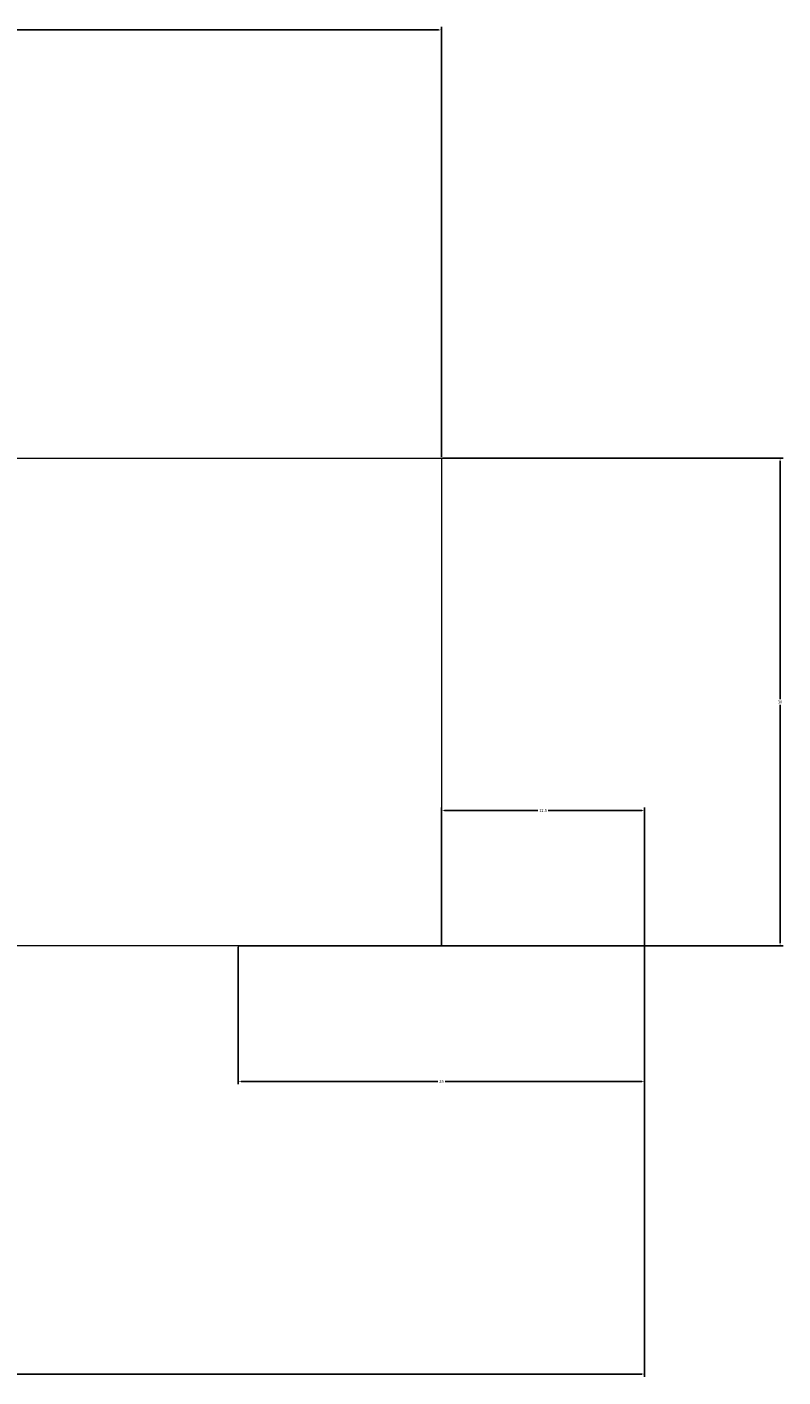
# Model space of a CAD drawing. Units: millimetres. Extents: x 2117 to 2298, y 1328 to 1411.
# Tile 3 of 3: x 2252 to 2298, y 1328 to 1411. Entities that reach past the tile are written whole.
import ezdxf

# ---------------------------------------------------------------- set-up
doc = ezdxf.new("R2010")
doc.units = ezdxf.units.MM
doc.layers.add('M-CONS', color=8, linetype='Continuous', lineweight=18)
doc.layers.add('M-DIMS', color=2, linetype='Continuous', lineweight=18)
doc.styles.get("Standard").update_dxf_attribs({"font": 'arial.ttf'})
doc.dimstyles.get("Standard").update_dxf_attribs({"dimtxt": 0.18, "dimasz": 0.18, "dimexe": 0.18, "dimexo": 0.0625, "dimgap": 0.09, "dimtad": 0, "dimtih": 1, "dimtoh": 1, "dimdec": 4, "dimzin": 0, "dimdsep": 46, "dimtxsty": 'Standard', "dimcen": 0.09, "dimadec": 0, "dimazin": 0, "dimtfac": 1, "dimtdec": 4, "dimtofl": 0, "dimtmove": 0, "dimatfit": 3, "dimfxl": 1, "dimtolj": 1, "dimtzin": 0, "dimarcsym": 0})

# ---------------------------------------------------------------- blocks, each defined once
blk = doc.blocks.new('*D7')
at = {"layer": 'Defpoints', "color": 0, "transparency": 16777216}
for p in [(2277.416, 1411.113), (2205.416, 1384.783), (2277.416, 1384.783)]:
    blk.add_point(p, dxfattribs=at)
at = {"layer": 'M-DIMS', "color": 0, "lineweight": -2, "transparency": 16777216}
for p, q in [((2205.416, 1384.845), (2205.416, 1411.293)), ((2205.596, 1411.113), (2241.199, 1411.113)), ((2277.236, 1411.113), (2241.633, 1411.113)), ((2277.416, 1384.845), (2277.416, 1411.293))]:
    blk.add_line(p, q, dxfattribs=at)
at = {"layer": 'M-DIMS', "color": 0, "transparency": 16777216}
for points in [[(2205.596, 1411.143), (2205.596, 1411.083), (2205.416, 1411.113)], [(2277.236, 1411.143), (2277.236, 1411.083), (2277.416, 1411.113)]]:
    blk.add_solid(points, dxfattribs=at)
at = {"layer": 'M-DIMS', "color": 0, "transparency": 16777216, "insert": (2241.416, 1411.113), "char_height": 0.18, "attachment_point": 5}
blk.add_mtext('\\A1;72', dxfattribs=at)
blk = doc.blocks.new('*D8')
at = {"layer": 'Defpoints', "color": 0, "transparency": 16777216}
for p in [(2289.916, 1363.113), (2277.416, 1354.783), (2289.916, 1354.783)]:
    blk.add_point(p, dxfattribs=at)
at = {"layer": 'M-DIMS', "color": 0, "lineweight": -2, "transparency": 16777216}
for p, q in [((2277.416, 1354.845), (2277.416, 1363.293)), ((2289.916, 1354.845), (2289.916, 1363.293)), ((2277.596, 1363.113), (2283.35, 1363.113)), ((2289.736, 1363.113), (2283.982, 1363.113))]:
    blk.add_line(p, q, dxfattribs=at)
at = {"layer": 'M-DIMS', "color": 0, "transparency": 16777216}
for points in [[(2277.596, 1363.143), (2277.596, 1363.083), (2277.416, 1363.113)], [(2289.736, 1363.143), (2289.736, 1363.083), (2289.916, 1363.113)]]:
    blk.add_solid(points, dxfattribs=at)
at = {"layer": 'M-DIMS', "color": 0, "transparency": 16777216, "insert": (2283.666, 1363.113), "char_height": 0.18, "attachment_point": 5}
blk.add_mtext('\\A1;12.5', dxfattribs=at)
blk = doc.blocks.new('*D10')
at = {"layer": 'Defpoints', "color": 0, "transparency": 16777216}
for p in [(2277.416, 1384.783), (2298.246, 1384.783), (2277.416, 1354.783)]:
    blk.add_point(p, dxfattribs=at)
at = {"layer": 'M-DIMS', "color": 0, "lineweight": -2, "transparency": 16777216}
for p, q in [((2277.479, 1384.783), (2298.426, 1384.783)), ((2298.246, 1384.603), (2298.246, 1369.965)), ((2298.246, 1354.963), (2298.246, 1369.601)), ((2277.479, 1354.783), (2298.426, 1354.783))]:
    blk.add_line(p, q, dxfattribs=at)
at = {"layer": 'M-DIMS', "color": 0, "transparency": 16777216}
for points in [[(2298.216, 1384.603), (2298.276, 1384.603), (2298.246, 1384.783)], [(2298.216, 1354.963), (2298.276, 1354.963), (2298.246, 1354.783)]]:
    blk.add_solid(points, dxfattribs=at)
at = {"layer": 'M-DIMS', "color": 0, "transparency": 16777216, "insert": (2298.246, 1369.783), "char_height": 0.18, "attachment_point": 5}
blk.add_mtext('\\A1;30', dxfattribs=at)
blk = doc.blocks.new('*D11')
at = {"layer": 'Defpoints', "color": 0, "transparency": 16777216}
for p in [(2264.916, 1354.783), (2289.916, 1354.783), (2264.916, 1346.453)]:
    blk.add_point(p, dxfattribs=at)
at = {"layer": 'M-DIMS', "color": 0, "lineweight": -2, "transparency": 16777216}
for p, q in [((2264.916, 1354.72), (2264.916, 1346.273)), ((2289.916, 1354.72), (2289.916, 1346.273)), ((2265.096, 1346.453), (2277.195, 1346.453)), ((2289.736, 1346.453), (2277.637, 1346.453))]:
    blk.add_line(p, q, dxfattribs=at)
at = {"layer": 'M-DIMS', "color": 0, "transparency": 16777216}
for points in [[(2265.096, 1346.483), (2265.096, 1346.423), (2264.916, 1346.453)], [(2289.736, 1346.483), (2289.736, 1346.423), (2289.916, 1346.453)]]:
    blk.add_solid(points, dxfattribs=at)
at = {"layer": 'M-DIMS', "color": 0, "transparency": 16777216, "insert": (2277.416, 1346.453), "char_height": 0.18, "attachment_point": 5}
blk.add_mtext('\\A1;25', dxfattribs=at)
blk = doc.blocks.new('*D12')
at = {"layer": 'Defpoints', "color": 0, "transparency": 16777216}
for p in [(2125.416, 1369.783), (2289.916, 1354.783), (2289.916, 1328.453)]:
    blk.add_point(p, dxfattribs=at)
at = {"layer": 'M-DIMS', "color": 0, "lineweight": -2, "transparency": 16777216}
for p, q in [((2125.416, 1369.72), (2125.416, 1328.273)), ((2289.916, 1354.72), (2289.916, 1328.273)), ((2125.596, 1328.453), (2207.28, 1328.453)), ((2289.736, 1328.453), (2208.052, 1328.453))]:
    blk.add_line(p, q, dxfattribs=at)
at = {"layer": 'M-DIMS', "color": 0, "transparency": 16777216}
for points in [[(2125.596, 1328.483), (2125.596, 1328.423), (2125.416, 1328.453)], [(2289.736, 1328.483), (2289.736, 1328.423), (2289.916, 1328.453)]]:
    blk.add_solid(points, dxfattribs=at)
at = {"layer": 'M-DIMS', "color": 0, "transparency": 16777216, "insert": (2207.666, 1328.453), "char_height": 0.18, "attachment_point": 5}
blk.add_mtext('\\A1;164.5', dxfattribs=at)

msp = doc.modelspace()

# ---------------------------------------------------------------- linework, layer by layer
at = {"layer": 'M-CONS'}
msp.add_lwpolyline([(2205.416, 1369.783), (2205.416, 1384.783), (2277.416, 1384.783), (2277.416, 1354.783), (2205.416, 1354.783)], dxfattribs=at)
at = {"layer": 'M-CONS', "extrusion": (0, -1, 0)}
msp.add_circle((2277.416, 28.5, -1354.783), 12.5, dxfattribs=at)

# ---------------------------------------------------------------- dimensions: what is measured, and where the dimension line sits
at = {"layer": 'M-DIMS'}
for base, p1, p2, override, picture, middle in [((2277.416, 1411.113), (2205.416, 1384.783), (2277.416, 1384.783), {"dimdec": 0, "dimlfac": 1, "dimrnd": 0, "dimzin": 0, "dimdsep": 46, "dimlunit": 2}, '*D7', (2241.416, 1411.113)), ((2289.916, 1328.453), (2125.416, 1369.783), (2289.916, 1354.783), {"dimdec": 1, "dimlfac": 1, "dimrnd": 0, "dimzin": 0, "dimdsep": 46, "dimlunit": 2}, '*D12', (2207.666, 1328.453)), ((2289.916, 1363.113), (2277.416, 1354.783), (2289.916, 1354.783), {"dimdec": 1, "dimlfac": 1, "dimrnd": 0, "dimzin": 0, "dimdsep": 46, "dimlunit": 2}, '*D8', (2283.666, 1363.113))]:
    dim = msp.add_linear_dim(base=base, p1=p1, p2=p2, dimstyle='Standard', override=override, dxfattribs=at)
    dim.commit()
    dim.dimension.update_dxf_attribs({"geometry": picture, "text_midpoint": middle})
for base, p1, p2, angle, picture, middle in [((2298.246, 1384.783), (2277.416, 1354.783), (2277.416, 1384.783), 90, '*D10', (2298.246, 1369.783)), ((2264.916, 1346.453), (2289.916, 1354.783), (2264.916, 1354.783), 180, '*D11', (2277.416, 1346.453))]:
    dim = msp.add_linear_dim(base=base, p1=p1, p2=p2, angle=angle, dimstyle='Standard', override={"dimdec": 0, "dimlfac": 1, "dimrnd": 0, "dimzin": 0, "dimdsep": 46, "dimlunit": 2}, dxfattribs=at)
    dim.commit()
    dim.dimension.update_dxf_attribs({"geometry": picture, "text_midpoint": middle})

doc.saveas('drawing.dxf')
